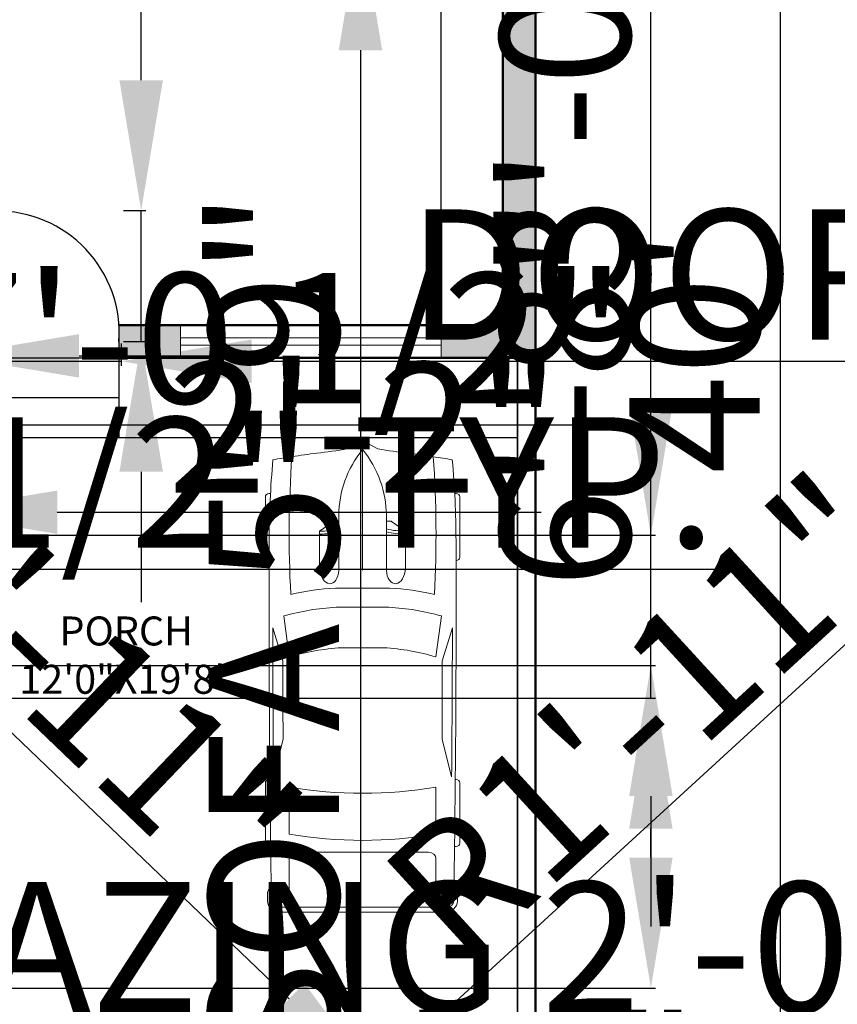
# Model space of a CAD drawing. Units: inches. Extents: x -299 to 1164, y -2 to 940.
# Tile 6 of 11: x 597 to 822, y 218 to 490. Entities that reach past the tile are written whole.
import ezdxf

# ---------------------------------------------------------------- set-up
doc = ezdxf.new("R2010")
doc.units = ezdxf.units.IN
for name, color, linetype, lineweight in [('A-AREA-IDEN', 3, 'Continuous', 25), ('C-SITE-VEHL', 8, 'Continuous', 13), ('C-SITE-WALL', 7, 'Continuous', 35), ('dimensions', 191, 'Continuous', 18), ('doors', 20, 'Continuous', 25), ('outer walls', 7, 'Continuous', 50), ('stairs', 6, 'Continuous', 25), ('windows', 130, 'Continuous', 18)]:
    doc.layers.add(name, color=color, linetype=linetype, lineweight=lineweight)
doc.layers.add('A-WALL-PATT', color=240, linetype='Continuous', lineweight=13, true_color=0xed1f24)
doc.styles.get("Standard").update_dxf_attribs({"font": 'arial.ttf'})
doc.dimstyles.new('ISO-25', dxfattribs={"dimtxt": 36, "dimasz": 36, "dimexe": 1.25, "dimexo": 0.625, "dimtad": 1, "dimlunit": 3, "dimtxsty": 'Standard', "dimcen": 2.5, "dimazin": 0, "dimtfac": 1, "dimtmove": 0, "dimatfit": 3, "dimfxl": 1, "dimarcsym": 0})

# ---------------------------------------------------------------- blocks, each defined once
blk = doc.blocks.new('*U11')
for p, q in [((536, 950.2), (536, 935.5)), ((1182.5, 987.8), (567.7, 987.8)), ((1214.1, 949.7), (1214.1, 950.2)), ((2234.8, 809.5), (1898.9, 912.4)), ((3411.6, 904.3), (3029.9, 807.2)), ((3440.5, 941.7), (3440.5, 950.2)), ((3472.1, 987.8), (4086.9, 987.8)), ((4118.5, 950.2), (4118.5, 934.1)), ((1778.8, 801), (2194.7, 745.5)), ((4736.4, -850.9), (4736.4, 850.9)), ((4785.3, -832.1), (4785.3, 832.1)), ((3515.9, 745.5), (3994.1, 745.5)), ((4736.4, 745.5), (4242, 745.5)), ((4178.7, 670.3), (4178.7, -670.3)), ((819.6, 295.3), (917.7, 436.1)), ((917.7, 436.1), (1293.8, 436.1)), ((756.2, 241.4), (1312.8, 241.4)), ((815.9, 241.4), (815.9, 283.3)), ((1496.5, -273.7), (1496.5, 273.7)), ((1690.4, -267.4), (1690.4, 267.4)), ((2101.5, 215.8), (2101.5, -215.8)), ((4736.4, -267.4), (4736.4, 267.4)), ((83, 155.7), (2.6, 10.3)), ((0, 0), (1312.8, 0)), ((2.6, -10.3), (83, -155.7)), ((756.2, -241.4), (1312.8, -241.4)), ((815.9, -241.4), (815.9, -283.3)), ((819.6, -295.3), (917.7, -436.1)), ((917.7, -436.1), (1293.8, -436.1)), ((2194.7, -745.5), (1778.8, -801)), ((3994.1, -745.5), (3515.9, -745.5)), ((4242, -745.5), (4736.4, -745.5)), ((2234.8, -809.5), (1898.9, -912.4)), ((3411.6, -904.3), (3029.9, -807.2)), ((536, -950.2), (536, -935.5)), ((1182.5, -987.8), (567.7, -987.8)), ((1214.1, -949.7), (1214.1, -950.2)), ((3440.5, -941.7), (3440.5, -950.2)), ((3472.1, -987.8), (4086.9, -987.8)), ((4118.5, -950.2), (4118.5, -934.1))]:
    blk.add_line(p, q)
for centre, major_axis, ratio, start_param, end_param in [((6757.2, -699.1), (0, 7958), 0.842304, 1.367076, 1.39176), ((1046.3, -12467.9), (0, 13417.1), 0.842304, 0.00281, 0.075598), ((567.7, 950.2), (0, -37.6), 0.842304, 3.141593, 4.712389), ((1637.8, -268112.7), (0, 269062.9), 0.842304, -0.013397, 0.002797), ((1182.5, 950.2), (0, 37.6), 0.842304, -1.570796, 0), ((1637.8, -268112.7), (0, -269025.3), 0.842304, 3.133765, 3.140441), ((3472.1, 950.2), (0, -37.6), 0.842304, 3.141593, 4.712389), ((4086.9, 950.2), (0, 37.6), 0.842304, -1.570796, 0), ((4588, 910.3), (0, 56.4), 0.842304, -0.013017, 1.249894), ((1637.8, -268131.5), (0, 269121), 0.842304, -0.013397, -0.013017), ((4673.1, 850.9), (0, -75.2), 0.842304, 1.570796, 3.128196), ((4673.1, 832.1), (0, -133.3), 0.842304, 1.570796, 3.128196), ((3436.4, 136.8), (0, 2077), 0.842304, 1.245306, 1.50788), ((2433, -93125.4), (0, -93935.2), 0.842304, 3.134049, 3.144098), ((6583, -699.1), (0, -7754.7), 0.842304, 4.528606, 4.561838), ((951.8, -15086.6), (0, -15832.5), 0.842304, 3.096046, 3.200911), ((3413.8, 136.8), (0, -2280.3), 0.842304, 4.449482, 4.652344), ((3799.7, 71.1), (0, -2021.3), 0.842304, 4.372215, 4.640744), ((433.9, 0), (0, 3734.3), 0.842304, 4.511394, 4.913384), ((912, 0), (0, 3734.3), 0.842304, 4.511394, 4.913384), ((4242, 670.3), (0, 75.2), 0.842304, 0, 1.570796), ((-5194.2, 1330.9), (0, -6374.4), 0.842304, 1.385369, 1.434372), ((331.1, 432), (0, 696.4), 0.842304, 4.435146, 4.718221), ((360.7, 432), (0, 696.4), 0.842304, 4.435146, 4.718221), ((1290.1, 338.8), (161, -9.1), 0.603834, -1.395552, 1.581315), ((756.2, -1185.2), (0, 1426.7), 0.842304, 0, 0.590319), ((831.8, 283.3), (0, 18.8), 0.842304, 0.879714, 1.570796), ((15.8, 0), (0, -18.8), 0.842304, 4.131459, 5.293319), ((756.2, 1185.2), (0, 1426.7), 0.842304, 2.551274, 3.141593), ((-5194.2, -1330.9), (0, 6374.4), 0.842304, -1.434372, -1.385369), ((831.8, -283.3), (0, -18.8), 0.842304, 4.712389, 5.403472), ((331.1, -432), (0, -696.4), 0.842304, 1.564964, 1.848039), ((360.7, -432), (0, -696.4), 0.842304, 1.564964, 1.848039), ((3413.8, -136.8), (0, -2280.3), 0.842304, -1.510751, -1.307889), ((3436.4, -136.8), (0, -2077), 0.842304, -1.50788, -1.245306), ((3799.7, -71.1), (0, -2021.3), 0.842304, -1.499151, -1.230623), ((6583, 699.1), (0, 7754.7), 0.842304, 1.721348, 1.754579), ((4242, -670.3), (0, -75.2), 0.842304, 4.712389, 6.283185), ((6757.2, 699.1), (0, 7958), 0.842304, 1.749832, 1.774517), ((951.8, 15086.6), (0, -15832.5), 0.842304, -0.059319, 0.045547), ((2433, 93125.4), (0, -93935.2), 0.842304, -0.002505, 0.007544), ((4673.1, -850.9), (0, 75.2), 0.842304, 3.15499, 4.712389), ((4673.1, -832.1), (0, -133.3), 0.842304, 0.013397, 1.570796), ((1046.3, 12467.9), (0, -13417.1), 0.842304, -0.075598, -0.00281), ((567.7, -950.2), (0, 37.6), 0.842304, 1.570796, 3.141593), ((1637.8, 268112.7), (0, 269062.9), 0.842304, 3.138796, 3.15499), ((1182.5, -950.2), (0, -37.6), 0.842304, 0, 1.570796), ((1637.8, 268112.7), (0, -269025.3), 0.842304, 0.001152, 0.007828), ((3472.1, -950.2), (0, -37.6), 0.842304, -1.570796, 0), ((4086.9, -950.2), (0, 37.6), 0.842304, 3.141593, 4.712389), ((4588, -910.3), (0, -56.4), 0.842304, -1.249894, 0.013017), ((1637.8, 268131.5), (0, 269121), 0.842304, 3.15461, 3.15499)]:
    blk.add_ellipse(centre, major_axis=major_axis, ratio=ratio, start_param=start_param, end_param=end_param)
at = {"extrusion": (0, 0, -1)}
blk.add_ellipse((1290.1, -338.8), major_axis=(161, 9.1), ratio=0.603834, start_param=-1.395552, end_param=1.581315, dxfattribs=at)
blk = doc.blocks.new('*D14')
at = {"layer": 'Defpoints', "color": 0, "transparency": 16777216}
for p in [(739.07, 638.49), (739.07, 158.49), (806.66, 158.49)]:
    blk.add_point(p, dxfattribs=at)
at = {"layer": 'dimensions', "color": 0, "lineweight": -2, "transparency": 16777216}
for p, q in [((739.7, 638.49), (807.91, 638.49)), ((806.66, 602.49), (806.66, 194.49)), ((739.7, 158.49), (807.91, 158.49))]:
    blk.add_line(p, q, dxfattribs=at)
at = {"layer": 'dimensions', "color": 0, "transparency": 16777216}
for points in [[(800.66, 602.49), (812.66, 602.49), (806.66, 638.49)], [(800.66, 194.49), (812.66, 194.49), (806.66, 158.49)]]:
    blk.add_solid(points, dxfattribs=at)
at = {"layer": 'dimensions', "color": 0, "transparency": 16777216, "insert": (787.65, 398.49), "char_height": 36, "attachment_point": 5, "rotation": 90}
blk.add_mtext("40'", dxfattribs=at)
blk = doc.blocks.new('WIN-72IN')
for p, q in [((0, 5.5), (72, 5.5)), ((0, 3.5), (72, 3.5))]:
    blk.add_line(p, q)
blk.add_lwpolyline([(0, 0), (72, 0), (72, 9), (0, 9)], close=True)
blk = doc.blocks.new('DOOR-36IN')
blk.add_lwpolyline([(0, 36), (2, 36), (2, 0), (0, 0)], close=True)
blk.add_arc((2.32, 2.25), 33.75, 356.1776, 90.5492)
blk = doc.blocks.new('*D23')
at = {"layer": 'Defpoints', "color": 0, "transparency": 16777216}
for p in [(701.12, 586.52), (690.74, 517.34), (701.12, 517.34)]:
    blk.add_point(p, dxfattribs=at)
at = {"layer": 'dimensions', "color": 0, "lineweight": -2, "transparency": 16777216}
for p, q in [((690.74, 622.52), (690.74, 658.52)), ((700.49, 586.52), (689.49, 586.52)), ((690.74, 586.52), (690.74, 517.34)), ((700.49, 517.34), (689.49, 517.34)), ((690.74, 481.34), (690.74, 197.66))]:
    blk.add_line(p, q, dxfattribs=at)
at = {"layer": 'dimensions', "color": 0, "transparency": 16777216}
for points in [[(684.74, 622.52), (696.74, 622.52), (690.74, 586.52)], [(684.74, 481.34), (696.74, 481.34), (690.74, 517.34)]]:
    blk.add_solid(points, dxfattribs=at)
at = {"layer": 'dimensions', "color": 0, "transparency": 16777216, "insert": (671.49, 321.5), "char_height": 36, "attachment_point": 5, "rotation": 90}
blk.add_mtext('SOFA 5\'-9"', dxfattribs=at)
blk = doc.blocks.new('*D28')
at = {"layer": 'Defpoints', "color": 0, "transparency": 16777216}
for p in [(379.74, 342.99), (412.07, 342.99), (412.07, 338.11)]:
    blk.add_point(p, dxfattribs=at)
at = {"layer": 'dimensions', "color": 0, "lineweight": -2, "transparency": 16777216}
for p, q in [((379.74, 342.36), (379.74, 336.86)), ((412.07, 342.36), (412.07, 336.86)), ((343.74, 338.11), (307.74, 338.11)), ((379.74, 338.11), (412.07, 338.11)), ((448.07, 338.11), (789.26, 338.11))]:
    blk.add_line(p, q, dxfattribs=at)
at = {"layer": 'dimensions', "color": 0, "transparency": 16777216}
for points in [[(343.74, 344.11), (343.74, 332.11), (379.74, 338.11)], [(448.07, 344.11), (448.07, 332.11), (412.07, 338.11)]]:
    blk.add_solid(points, dxfattribs=at)
at = {"layer": 'dimensions', "color": 0, "transparency": 16777216, "insert": (636.66, 357.35), "char_height": 36, "attachment_point": 5}
blk.add_mtext('2\'-8 1/2" TYP.', dxfattribs=at)
blk = doc.blocks.new('*D29')
at = {"layer": 'Defpoints', "color": 0, "transparency": 16777216}
for p in [(304.07, 183.49), (376.07, 183.49), (376.07, 172.69)]:
    blk.add_point(p, dxfattribs=at)
at = {"layer": 'dimensions', "color": 0, "lineweight": -2, "transparency": 16777216}
for p, q in [((304.07, 182.86), (304.07, 171.44)), ((376.07, 182.86), (376.07, 171.44)), ((268.07, 172.69), (232.07, 172.69)), ((304.07, 172.69), (376.07, 172.69)), ((412.07, 172.69), (904.87, 172.69))]:
    blk.add_line(p, q, dxfattribs=at)
at = {"layer": 'dimensions', "color": 0, "transparency": 16777216}
for points in [[(268.07, 178.69), (268.07, 166.69), (304.07, 172.69)], [(412.07, 178.69), (412.07, 166.69), (376.07, 172.69)]]:
    blk.add_solid(points, dxfattribs=at)
at = {"layer": 'dimensions', "color": 0, "transparency": 16777216, "insert": (676.47, 191.94), "char_height": 36, "attachment_point": 5}
blk.add_mtext('WINDOW 6\'-0" TYP.', dxfattribs=at)
blk = doc.blocks.new('*D33')
at = {"layer": 'Defpoints', "color": 0, "transparency": 16777216}
for p in [(419.84, 213.49), (443.84, 213.49), (443.84, 209.89)]:
    blk.add_point(p, dxfattribs=at)
at = {"layer": 'dimensions', "color": 0, "lineweight": -2, "transparency": 16777216}
for p, q in [((419.84, 212.86), (419.84, 208.64)), ((443.84, 212.86), (443.84, 208.64)), ((383.84, 209.89), (347.84, 209.89)), ((419.84, 209.89), (443.84, 209.89)), ((479.84, 209.89), (970.68, 209.89))]:
    blk.add_line(p, q, dxfattribs=at)
at = {"layer": 'dimensions', "color": 0, "transparency": 16777216}
for points in [[(383.84, 215.89), (383.84, 203.89), (419.84, 209.89)], [(479.84, 215.89), (479.84, 203.89), (443.84, 209.89)]]:
    blk.add_solid(points, dxfattribs=at)
at = {"layer": 'dimensions', "color": 0, "transparency": 16777216, "insert": (743.26, 229.13), "char_height": 36, "attachment_point": 5}
blk.add_mtext('GLAZING 2\'-0" TYP.', dxfattribs=at)
blk = doc.blocks.new('*D35')
at = {"layer": 'Defpoints', "color": 0, "transparency": 16777216}
for p in [(307.07, 495.34), (268.07, 489.49), (307.07, 489.49)]:
    blk.add_point(p, dxfattribs=at)
at = {"layer": 'dimensions', "color": 0, "lineweight": -2, "transparency": 16777216}
for p, q in [((232.07, 495.34), (196.07, 495.34)), ((268.07, 490.11), (268.07, 496.59)), ((268.07, 495.34), (307.07, 495.34)), ((307.07, 490.11), (307.07, 496.59)), ((343.07, 495.34), (749.73, 495.34))]:
    blk.add_line(p, q, dxfattribs=at)
at = {"layer": 'dimensions', "color": 0, "transparency": 16777216}
for points in [[(232.07, 501.34), (232.07, 489.34), (268.07, 495.34)], [(343.07, 501.34), (343.07, 489.34), (307.07, 495.34)]]:
    blk.add_solid(points, dxfattribs=at)
at = {"layer": 'dimensions', "color": 0, "transparency": 16777216, "insert": (564.4, 514.36), "char_height": 36, "attachment_point": 5}
blk.add_mtext('VENT 3\'-3" TYP.', dxfattribs=at)
blk = doc.blocks.new('*D37')
at = {"layer": 'Defpoints', "color": 0, "transparency": 16777216}
for p in [(588.07, 400.99), (624.7, 400.99), (624.7, 395.5)]:
    blk.add_point(p, dxfattribs=at)
at = {"layer": 'dimensions', "color": 0, "lineweight": -2, "transparency": 16777216}
for p, q in [((588.07, 400.36), (588.07, 394.25)), ((624.7, 400.36), (624.7, 394.25)), ((552.07, 395.5), (516.07, 395.5)), ((588.07, 395.5), (624.7, 395.5)), ((660.7, 395.5), (1164.33, 395.5))]:
    blk.add_line(p, q, dxfattribs=at)
at = {"layer": 'dimensions', "color": 0, "transparency": 16777216}
for points in [[(552.07, 401.5), (552.07, 389.5), (588.07, 395.5)], [(660.7, 401.5), (660.7, 389.5), (624.7, 395.5)]]:
    blk.add_solid(points, dxfattribs=at)
at = {"layer": 'dimensions', "color": 0, "transparency": 16777216, "insert": (930.51, 414.76), "char_height": 36, "attachment_point": 5}
blk.add_mtext('DOOR 3\'-0 1/2" TYP.', dxfattribs=at)
blk = doc.blocks.new('*D38')
at = {"layer": 'Defpoints', "color": 0, "transparency": 16777216}
for p in [(624.7, 437.08), (630.19, 437.08), (624.7, 400.99)]:
    blk.add_point(p, dxfattribs=at)
at = {"layer": 'dimensions', "color": 0, "lineweight": -2, "transparency": 16777216}
for p, q in [((630.19, 473.08), (630.19, 729.74)), ((625.32, 437.08), (631.44, 437.08)), ((630.19, 400.99), (630.19, 437.08)), ((625.32, 400.99), (631.44, 400.99)), ((630.19, 364.99), (630.19, 328.99))]:
    blk.add_line(p, q, dxfattribs=at)
at = {"layer": 'dimensions', "color": 0, "transparency": 16777216}
for points in [[(624.19, 473.08), (636.19, 473.08), (630.19, 437.08)], [(624.19, 364.99), (636.19, 364.99), (630.19, 400.99)]]:
    blk.add_solid(points, dxfattribs=at)
at = {"layer": 'dimensions', "color": 0, "transparency": 16777216, "insert": (611.17, 619.41), "char_height": 36, "attachment_point": 5, "rotation": 90}
blk.add_mtext('3\'-0" TYP.', dxfattribs=at)
blk = doc.blocks.new('*D39')
at = {"layer": 'Defpoints', "color": 0, "transparency": 16777216}
for p in [(575.6, 509.45), (484.6, 495.8), (575.6, 495.8)]:
    blk.add_point(p, dxfattribs=at)
at = {"layer": 'dimensions', "color": 0, "lineweight": -2, "transparency": 16777216}
for p, q in [((484.6, 496.43), (484.6, 510.7)), ((520.6, 509.45), (539.6, 509.45)), ((575.6, 496.43), (575.6, 510.7)), ((575.6, 509.45), (1008.53, 509.45))]:
    blk.add_line(p, q, dxfattribs=at)
at = {"layer": 'dimensions', "color": 0, "transparency": 16777216}
for points in [[(520.6, 515.45), (520.6, 503.45), (484.6, 509.45)], [(539.6, 515.45), (539.6, 503.45), (575.6, 509.45)]]:
    blk.add_solid(points, dxfattribs=at)
at = {"layer": 'dimensions', "color": 0, "transparency": 16777216, "insert": (810.07, 528.69), "char_height": 36, "attachment_point": 5}
blk.add_mtext('DINING SET 7\'-7"', dxfattribs=at)
blk = doc.blocks.new('*D42')
at = {"layer": 'Defpoints', "color": 0, "transparency": 16777216}
for p in [(545.04, 358.33), (571.04, 358.33), (571.04, 353.83)]:
    blk.add_point(p, dxfattribs=at)
at = {"layer": 'dimensions', "color": 0, "lineweight": -2, "transparency": 16777216}
for p, q in [((545.04, 357.71), (545.04, 352.58)), ((571.04, 357.71), (571.04, 352.58)), ((509.04, 353.83), (473.04, 353.83)), ((545.04, 353.83), (571.04, 353.83)), ((607.04, 353.83), (740.6, 353.83))]:
    blk.add_line(p, q, dxfattribs=at)
at = {"layer": 'dimensions', "color": 0, "transparency": 16777216}
for points in [[(509.04, 359.83), (509.04, 347.83), (545.04, 353.83)], [(607.04, 359.83), (607.04, 347.83), (571.04, 353.83)]]:
    blk.add_solid(points, dxfattribs=at)
at = {"layer": 'dimensions', "color": 0, "transparency": 16777216, "insert": (691.82, 372.53), "char_height": 36, "attachment_point": 5}
blk.add_mtext('2\'-2"', dxfattribs=at)
blk = doc.blocks.new('*D46')
at = {"layer": 'Defpoints', "color": 0, "transparency": 16777216}
for p in [(579.07, 302.49), (770.93, 302.49), (579.07, 222.49)]:
    blk.add_point(p, dxfattribs=at)
at = {"layer": 'dimensions', "color": 0, "lineweight": -2, "transparency": 16777216}
for p, q in [((770.93, 302.49), (770.93, 435.63)), ((579.7, 302.49), (772.18, 302.49)), ((770.93, 258.49), (770.93, 266.49)), ((579.7, 222.49), (772.18, 222.49))]:
    blk.add_line(p, q, dxfattribs=at)
at = {"layer": 'dimensions', "color": 0, "transparency": 16777216}
for points in [[(764.93, 266.49), (776.93, 266.49), (770.93, 302.49)], [(764.93, 258.49), (776.93, 258.49), (770.93, 222.49)]]:
    blk.add_solid(points, dxfattribs=at)
at = {"layer": 'dimensions', "color": 0, "transparency": 16777216, "insert": (751.92, 387.06), "char_height": 36, "attachment_point": 5, "rotation": 90}
blk.add_mtext('6\'-8"', dxfattribs=at)
blk = doc.blocks.new('*D47')
at = {"layer": 'Defpoints', "color": 0, "transparency": 16777216}
for p in [(502.07, 668.99), (466.07, 222.49), (502.07, 222.49)]:
    blk.add_point(p, dxfattribs=at)
at = {"layer": 'dimensions', "color": 0, "lineweight": -2, "transparency": 16777216}
for p, q in [((430.07, 668.99), (394.07, 668.99)), ((466.07, 223.11), (466.07, 670.24)), ((466.07, 668.99), (502.07, 668.99)), ((502.07, 223.11), (502.07, 670.24)), ((538.07, 668.99), (670.99, 668.99))]:
    blk.add_line(p, q, dxfattribs=at)
at = {"layer": 'dimensions', "color": 0, "transparency": 16777216}
for points in [[(430.07, 674.99), (430.07, 662.99), (466.07, 668.99)], [(538.07, 674.99), (538.07, 662.99), (502.07, 668.99)]]:
    blk.add_solid(points, dxfattribs=at)
at = {"layer": 'dimensions', "color": 0, "transparency": 16777216, "insert": (622.53, 688.01), "char_height": 36, "attachment_point": 5}
blk.add_mtext('3\'-0"', dxfattribs=at)
blk = doc.blocks.new('*D48')
at = {"layer": 'Defpoints', "color": 0, "transparency": 16777216}
for p in [(546.07, 668.99), (535.07, 222.49), (546.07, 222.49)]:
    blk.add_point(p, dxfattribs=at)
at = {"layer": 'dimensions', "color": 0, "lineweight": -2, "transparency": 16777216}
for p, q in [((499.07, 668.99), (463.07, 668.99)), ((535.07, 223.11), (535.07, 670.24)), ((535.07, 668.99), (546.07, 668.99)), ((546.07, 223.11), (546.07, 670.24)), ((582.07, 668.99), (742.99, 668.99))]:
    blk.add_line(p, q, dxfattribs=at)
at = {"layer": 'dimensions', "color": 0, "transparency": 16777216}
for points in [[(499.07, 674.99), (499.07, 662.99), (535.07, 668.99)], [(582.07, 674.99), (582.07, 662.99), (546.07, 668.99)]]:
    blk.add_solid(points, dxfattribs=at)
at = {"layer": 'dimensions', "color": 0, "transparency": 16777216, "insert": (680.53, 687.99), "char_height": 36, "attachment_point": 5}
blk.add_mtext('0\'-11"', dxfattribs=at)
blk = doc.blocks.new('*D51')
at = {"layer": 'Defpoints', "color": 0, "transparency": 16777216}
for p in [(739.07, 668.99), (713.07, 405.49), (739.07, 396.49)]:
    blk.add_point(p, dxfattribs=at)
at = {"layer": 'dimensions', "color": 0, "lineweight": -2, "transparency": 16777216}
for p, q in [((677.07, 668.99), (641.07, 668.99)), ((713.07, 406.11), (713.07, 670.24)), ((713.07, 668.99), (739.07, 668.99)), ((739.07, 397.11), (739.07, 670.24)), ((775.07, 668.99), (908.63, 668.99))]:
    blk.add_line(p, q, dxfattribs=at)
at = {"layer": 'dimensions', "color": 0, "transparency": 16777216}
for points in [[(677.07, 674.99), (677.07, 662.99), (713.07, 668.99)], [(775.07, 674.99), (775.07, 662.99), (739.07, 668.99)]]:
    blk.add_solid(points, dxfattribs=at)
at = {"layer": 'dimensions', "color": 0, "transparency": 16777216, "insert": (859.85, 687.69), "char_height": 36, "attachment_point": 5}
blk.add_mtext('2\'-2"', dxfattribs=at)
blk = doc.blocks.new('*D52')
at = {"layer": 'Defpoints', "color": 0, "transparency": 16777216}
for p in [(575.54, 668.99), (527.54, 311.49), (575.54, 311.49)]:
    blk.add_point(p, dxfattribs=at)
at = {"layer": 'dimensions', "color": 0, "lineweight": -2, "transparency": 16777216}
for p, q in [((491.54, 668.99), (455.54, 668.99)), ((527.54, 312.11), (527.54, 670.24)), ((527.54, 668.99), (575.54, 668.99)), ((575.54, 312.11), (575.54, 670.24)), ((611.54, 668.99), (745.94, 668.99))]:
    blk.add_line(p, q, dxfattribs=at)
at = {"layer": 'dimensions', "color": 0, "transparency": 16777216}
for points in [[(491.54, 674.99), (491.54, 662.99), (527.54, 668.99)], [(611.54, 674.99), (611.54, 662.99), (575.54, 668.99)]]:
    blk.add_solid(points, dxfattribs=at)
at = {"layer": 'dimensions', "color": 0, "transparency": 16777216, "insert": (696.74, 687.99), "char_height": 36, "attachment_point": 5}
blk.add_mtext('4\'-0"', dxfattribs=at)
blk = doc.blocks.new('*D56')
at = {"layer": 'Defpoints', "color": 0, "transparency": 16777216}
for p in [(541.07, 377.99), (456.35, 347.49), (541.07, 347.49)]:
    blk.add_point(p, dxfattribs=at)
at = {"layer": 'dimensions', "color": 0, "lineweight": -2, "transparency": 16777216}
for p, q in [((456.35, 348.11), (456.35, 379.24)), ((492.35, 377.99), (505.07, 377.99)), ((541.07, 348.11), (541.07, 379.24)), ((541.07, 377.99), (757.61, 377.99))]:
    blk.add_line(p, q, dxfattribs=at)
at = {"layer": 'dimensions', "color": 0, "transparency": 16777216}
for points in [[(492.35, 383.99), (492.35, 371.99), (456.35, 377.99)], [(505.07, 383.99), (505.07, 371.99), (541.07, 377.99)]]:
    blk.add_solid(points, dxfattribs=at)
at = {"layer": 'dimensions', "color": 0, "transparency": 16777216, "insert": (667.34, 397.23), "char_height": 36, "attachment_point": 5}
blk.add_mtext('7\'-0 1/2"', dxfattribs=at)
blk = doc.blocks.new('*D57')
at = {"layer": 'Defpoints', "color": 0, "transparency": 16777216}
for p in [(541.07, 427.49), (577.07, 427.49), (541.07, 396.99)]:
    blk.add_point(p, dxfattribs=at)
at = {"layer": 'dimensions', "color": 0, "lineweight": -2, "transparency": 16777216}
for p, q in [((541.07, 426.86), (541.07, 395.74)), ((577.07, 426.86), (577.07, 395.74)), ((505.07, 396.99), (372.15, 396.99)), ((577.07, 396.99), (541.07, 396.99)), ((613.07, 396.99), (649.07, 396.99))]:
    blk.add_line(p, q, dxfattribs=at)
at = {"layer": 'dimensions', "color": 0, "transparency": 16777216}
for points in [[(505.07, 402.99), (505.07, 390.99), (541.07, 396.99)], [(613.07, 402.99), (613.07, 390.99), (577.07, 396.99)]]:
    blk.add_solid(points, dxfattribs=at)
at = {"layer": 'dimensions', "color": 0, "transparency": 16777216, "insert": (420.61, 416.01), "char_height": 36, "attachment_point": 5}
blk.add_mtext('3\'-0"', dxfattribs=at)
blk = doc.blocks.new('*D58')
at = {"layer": 'Defpoints', "color": 0, "transparency": 16777216}
for p in [(456.35, 347.49), (770.93, 347.49), (456.35, 311.49)]:
    blk.add_point(p, dxfattribs=at)
at = {"layer": 'dimensions', "color": 0, "lineweight": -2, "transparency": 16777216}
for p, q in [((770.93, 383.49), (770.93, 516.41)), ((456.97, 347.49), (772.18, 347.49)), ((770.93, 311.49), (770.93, 347.49)), ((456.97, 311.49), (772.18, 311.49)), ((770.93, 275.49), (770.93, 239.49))]:
    blk.add_line(p, q, dxfattribs=at)
at = {"layer": 'dimensions', "color": 0, "transparency": 16777216}
for points in [[(764.93, 383.49), (776.93, 383.49), (770.93, 347.49)], [(764.93, 275.49), (776.93, 275.49), (770.93, 311.49)]]:
    blk.add_solid(points, dxfattribs=at)
at = {"layer": 'dimensions', "color": 0, "transparency": 16777216, "insert": (751.91, 467.95), "char_height": 36, "attachment_point": 5, "rotation": 90}
blk.add_mtext('3\'-0"', dxfattribs=at)
blk = doc.blocks.new('*D59')
at = {"layer": 'Defpoints', "color": 0, "transparency": 16777216}
for p in [(697.05, 194.59), (730.81, 162.24)]:
    blk.add_point(p, dxfattribs=at)
at = {"layer": 'dimensions', "color": 0, "lineweight": -2, "transparency": 16777216}
for p, q in [((530.01, 354.68), (671.06, 219.5)), ((730.81, 162.24), (697.05, 194.59))]:
    blk.add_line(p, q, dxfattribs=at)
at = {"layer": 'dimensions', "color": 0, "transparency": 16777216}
blk.add_solid([(675.21, 223.83), (666.91, 215.17), (697.05, 194.59)], dxfattribs=at)
at = {"layer": 'dimensions', "color": 0, "transparency": 16777216, "insert": (600.7, 313.27), "char_height": 36, "attachment_point": 5, "rotation": 316.2186}
blk.add_mtext('R3\'-11"', dxfattribs=at)
blk = doc.blocks.new('*D60')
at = {"layer": 'Defpoints', "color": 0, "transparency": 16777216}
for p in [(672.12, 177.62), (655.34, 162.24)]:
    blk.add_point(p, dxfattribs=at)
at = {"layer": 'dimensions', "color": 0, "lineweight": -2, "transparency": 16777216}
for p, q in [((842.68, 333.96), (698.66, 201.95)), ((655.34, 162.24), (672.12, 177.62))]:
    blk.add_line(p, q, dxfattribs=at)
at = {"layer": 'dimensions', "color": 0, "transparency": 16777216}
blk.add_solid([(694.61, 206.37), (702.71, 197.52), (672.12, 177.62)], dxfattribs=at)
at = {"layer": 'dimensions', "color": 0, "transparency": 16777216, "insert": (771.3, 293.9), "char_height": 36, "attachment_point": 5, "rotation": 42.5105}
blk.add_mtext('R1\'-11"', dxfattribs=at)
blk = doc.blocks.new('*D62')
at = {"layer": 'Defpoints', "color": 0, "transparency": 16777216}
for p in [(420.34, 307.74), (441.36, 288.12)]:
    blk.add_point(p, dxfattribs=at)
at = {"layer": 'dimensions', "color": 0, "lineweight": -2, "transparency": 16777216}
for p, q in [((420.34, 307.74), (441.36, 288.12)), ((646.59, 96.57), (467.68, 263.55))]:
    blk.add_line(p, q, dxfattribs=at)
at = {"layer": 'dimensions', "color": 0, "transparency": 16777216}
blk.add_solid([(471.78, 267.94), (463.59, 259.17), (441.36, 288.12)], dxfattribs=at)
at = {"layer": 'dimensions', "color": 0, "transparency": 16777216, "insert": (583.27, 181.68), "char_height": 36, "attachment_point": 5, "rotation": 316.9755}
blk.add_mtext('3X R2\'-5"', dxfattribs=at)

msp = doc.modelspace()

# ---------------------------------------------------------------- hatches: boundary and pattern name
at = {"layer": 'A-WALL-PATT'}
h = msp.add_hatch(color=256, dxfattribs=at)
h.dxf.hatch_style = 1
h.paths.add_polyline_path([(312.071, 460.489), (307.071, 460.489), (307.071, 432.489), (307.071, 427.489), (372.071, 427.489), (372.071, 375.489), (372.071, 370.489), (380.071, 370.489, -0.0217424), (380.071, 372.989), (380.071, 375.489), (377.071, 375.489), (377.071, 427.489), (417.071, 427.489), (417.071, 489.489), (412.071, 489.489), (412.071, 484.489), (412.071, 432.489), (312.071, 432.489)], flags=17)
h.paths.add_polyline_path([(340.071, 372.989, -0.0217424), (340.071, 375.489), (268.071, 375.489), (268.071, 427.489), (268.071, 432.489), (268.071, 484.489), (268.071, 489.489), (268.071, 629.489), (412.071, 629.489), (412.071, 527.563, -0.0185322), (414.571, 527.489), (417.071, 527.489), (417.071, 629.489), (581.071, 629.489), (581.071, 553.489), (586.071, 553.489), (586.071, 629.489), (730.071, 629.489), (730.071, 405.489), (713.071, 405.489), (713.071, 396.489), (739.071, 396.489), (739.071, 638.489), (259.071, 638.489), (259.071, 183.489), (304.071, 183.489), (304.071, 192.489), (268.071, 192.489), (268.071, 370.489), (340.071, 370.489)])
h.paths.add_polyline_path([(417.071, 188.489), (417.071, 213.489), (461.071, 213.489), (461.071, 188.489)], flags=16)
h.paths.add_polyline_path([(586.071, 313.578), (577.071, 313.578), (577.071, 311.489), (575.54, 311.489), (575.54, 302.489), (586.071, 302.489)], flags=16)
h.paths.add_polyline_path([(586.071, 405.489), (586.071, 481.489), (581.071, 481.489), (581.071, 432.489), (499.071, 432.489), (499.071, 427.489), (577.071, 427.489), (577.071, 385.578), (586.071, 385.578), (586.071, 396.489)], flags=17)
h.paths.add_polyline_path([(641.071, 405.489), (624.071, 405.489, -0.0333689), (624.071, 400.989), (624.071, 396.489), (641.071, 396.489)], flags=17)
h.paths.add_polyline_path([(491.866, 222.489), (491.866, 213.489), (586.071, 213.489), (586.071, 222.489)])
edge = h.paths.add_edge_path()
edge.add_line((467.866, 213.489), (467.866, 222.489))
edge.add_line((467.866, 222.489), (466.071, 222.489))
edge.add_line((466.071, 222.489), (466.071, 302.489))
edge.add_line((466.071, 302.489), (527.54, 302.489))
edge.add_line((527.54, 302.489), (527.54, 311.489))
edge.add_line((527.54, 311.489), (449.071, 311.489))
edge.add_line((449.071, 311.489), (449.071, 308.989))
edge.add_arc((420.339, 307.739), 28.759, -2.4911, 2.4911, ccw=False)
edge.add_line((449.071, 306.489), (461.071, 306.489))
edge.add_line((461.071, 306.489), (461.071, 222.489))
edge.add_line((461.071, 222.489), (443.844, 222.489))
edge.add_line((443.844, 222.489), (443.844, 213.489))
edge.add_line((443.844, 213.489), (419.844, 213.489))
edge.add_line((419.844, 213.489), (419.844, 222.489))
edge.add_line((419.844, 222.489), (417.071, 222.489))
edge.add_line((417.071, 222.489), (417.071, 306.489))
edge.add_line((417.071, 306.489), (417.071, 311.489))
edge.add_line((417.071, 311.489), (417.071, 375.489))
edge.add_line((417.071, 375.489), (412.071, 375.489))
edge.add_line((412.071, 375.489), (412.071, 370.489))
edge.add_line((412.071, 370.489), (412.071, 192.489))
edge.add_line((412.071, 192.489), (376.071, 192.489))
edge.add_line((376.071, 192.489), (376.071, 183.489))
edge.add_line((376.071, 183.489), (412.071, 183.489))
edge.add_line((412.071, 183.489), (466.071, 183.489))
edge.add_line((466.071, 183.489), (466.071, 213.489))
edge.add_line((466.071, 213.489), (467.866, 213.489))

# ---------------------------------------------------------------- linework, layer by layer
at = {"layer": 'C-SITE-WALL'}
msp.add_line((734.071, 163.489), (734.071, 396.489), dxfattribs=at)
at = {"layer": 'doors'}
msp.add_line((624.071, 405.489), (624.071, 396.489), dxfattribs=at)
at = {"layer": 'outer walls'}
for p, q in [((739.071, 158.489), (739.071, 638.489)), ((730.071, 405.489), (730.071, 629.489)), ((730.071, 405.489), (624.071, 405.489)), ((739.071, 396.489), (624.071, 396.489))]:
    msp.add_line(p, q, dxfattribs=at)
at = {"layer": 'stairs'}
for p, q in [((588.071, 396.489), (624.071, 396.489)), ((624.071, 396.489), (624.071, 374.489)), ((586.071, 385.489), (624.071, 385.489)), ((586.071, 374.489), (624.071, 374.489)), ((624.071, 374.489), (734.071, 374.489))]:
    msp.add_line(p, q, dxfattribs=at)

# ---------------------------------------------------------------- block references
at = {"layer": 'C-SITE-VEHL', "xscale": 0.0271817845741683, "yscale": 0.0271817845741683, "zscale": 0.0271817845741683, "rotation": 270}
msp.add_blockref('*U11', (691.331, 373.539), dxfattribs=at)
at = {"layer": 'doors'}
msp.add_blockref('DOOR-36IN', (588.071, 400.989), dxfattribs=at)
at = {"layer": 'windows'}
msp.add_blockref('WIN-72IN', (641.071, 396.489), dxfattribs=at)

# ---------------------------------------------------------------- texts
at = {"layer": 'A-AREA-IDEN', "insert": (591.141, 325.046), "char_height": 8, "attachment_point": 1}
msp.add_mtext_dynamic_manual_height_columns('\\pxqc,t15;PORCH\\P12\'0"X19\'8"', width=69.83809, gutter_width=12.5, heights=[0], dxfattribs=at)

# ---------------------------------------------------------------- dimensions: what is measured, and where the dimension line sits
at = {"layer": 'dimensions'}
for base, p1, p2, angle, text, picture, middle in [((630.192, 437.079), (624.698, 400.989), (624.698, 437.079), 90, '<> TYP.', '*D38', (611.174, 619.411)), ((690.742, 517.338), (701.119, 586.518), (701.119, 517.338), 270, 'SOFA <>', '*D23', (671.49, 321.5))]:
    dim = msp.add_linear_dim(base=base, p1=p1, p2=p2, angle=angle, text=text, dimstyle='ISO-25', override={"dimdec": 1, "dimlfac": 1, "dimrnd": 0, "dimzin": 1, "dimdsep": 46, "dimlunit": 4, "dimfrac": 2}, dxfattribs=at)
    dim.commit()
    dim.dimension.update_dxf_attribs({"geometry": picture, "text_midpoint": middle})
for base, p1, p2, picture, middle in [((502.071, 668.989), (466.071, 222.489), (502.071, 222.489), '*D47', (622.532, 688.007)), ((575.54, 668.989), (527.54, 311.489), (575.54, 311.489), '*D52', (696.738, 687.995)), ((546.071, 668.989), (535.071, 222.489), (546.071, 222.489), '*D48', (680.53, 687.995)), ((739.071, 668.989), (713.071, 405.489), (739.071, 396.489), '*D51', (859.852, 687.688)), ((541.071, 377.989), (456.348, 347.489), (541.071, 347.489), '*D56', (667.34, 397.228)), ((571.036, 353.835), (545.036, 358.335), (571.036, 358.335), '*D42', (691.817, 372.534))]:
    dim = msp.add_linear_dim(base=base, p1=p1, p2=p2, dimstyle='ISO-25', override={"dimdec": 1, "dimlfac": 1, "dimrnd": 0, "dimzin": 1, "dimdsep": 46, "dimlunit": 4, "dimfrac": 2}, dxfattribs=at)
    dim.commit()
    dim.dimension.update_dxf_attribs({"geometry": picture, "text_midpoint": middle})
for base, p1, p2, angle, override, picture, middle in [((806.659, 158.489), (739.071, 638.489), (739.071, 158.489), 90, {"dimclrd": 0, "dimclre": 0, "dimclrt": 0}, '*D14', (787.654, 398.489)), ((770.929, 347.489), (456.348, 311.489), (456.348, 347.489), 90, {"dimdec": 1, "dimlfac": 1, "dimrnd": 0, "dimzin": 1, "dimdsep": 46, "dimlunit": 4, "dimfrac": 2}, '*D58', (751.911, 467.95)), ((541.071, 396.989), (577.071, 427.489), (541.071, 427.489), 180, {"dimdec": 1, "dimlfac": 1, "dimrnd": 0, "dimzin": 1, "dimdsep": 46, "dimlunit": 4, "dimfrac": 2}, '*D57', (420.61, 416.007)), ((770.929, 302.489), (579.071, 222.489), (579.071, 302.489), 90, {"dimdec": 1, "dimlfac": 1, "dimrnd": 0, "dimzin": 1, "dimdsep": 46, "dimlunit": 4, "dimfrac": 2}, '*D46', (751.923, 387.061))]:
    dim = msp.add_linear_dim(base=base, p1=p1, p2=p2, angle=angle, dimstyle='ISO-25', override=override, dxfattribs=at)
    dim.commit()
    dim.dimension.update_dxf_attribs({"geometry": picture, "text_midpoint": middle})
for base, p1, p2, text, picture, middle in [((575.6, 509.45), (484.6, 495.8), (575.6, 495.8), 'DINING SET <>', '*D39', (810.066, 528.689)), ((307.071, 495.339), (268.071, 489.489), (307.071, 489.489), 'VENT <> TYP.', '*D35', (564.399, 514.357)), ((624.698, 395.495), (588.071, 400.989), (624.698, 400.989), 'DOOR <> TYP.', '*D37', (930.512, 414.759)), ((412.071, 338.114), (379.736, 342.989), (412.071, 342.989), '<> TYP.', '*D28', (636.665, 357.353)), ((443.844, 209.889), (419.844, 213.489), (443.844, 213.489), 'GLAZING <> TYP.', '*D33', (743.261, 229.128)), ((376.071, 172.689), (304.071, 183.489), (376.071, 183.489), 'WINDOW <> TYP.', '*D29', (676.471, 191.94))]:
    dim = msp.add_linear_dim(base=base, p1=p1, p2=p2, text=text, dimstyle='ISO-25', override={"dimdec": 1, "dimlfac": 1, "dimrnd": 0, "dimzin": 1, "dimdsep": 46, "dimlunit": 4, "dimfrac": 2}, dxfattribs=at)
    dim.commit()
    dim.dimension.update_dxf_attribs({"geometry": picture, "text_midpoint": middle})
for center, mpoint, picture, middle in [((730.81, 162.239), (697.053, 194.59), '*D59', (600.698, 313.273)), ((655.344, 162.239), (672.123, 177.62), '*D60', (771.303, 293.901))]:
    dim = msp.add_radius_dim(center=center, mpoint=mpoint, dimstyle='ISO-25', override={"dimdec": 1, "dimlfac": 1, "dimrnd": 0, "dimzin": 1, "dimdsep": 46, "dimlunit": 4, "dimfrac": 2}, dxfattribs=at)
    dim.commit()
    dim.dimension.update_dxf_attribs({"geometry": picture, "text_midpoint": middle})
dim = msp.add_radius_dim(center=(420.339, 307.739), mpoint=(441.364, 288.116), text='3X <>', dimstyle='ISO-25', override={"dimdec": 1, "dimlfac": 1, "dimrnd": 0, "dimzin": 1, "dimdsep": 46, "dimlunit": 4, "dimfrac": 2}, dxfattribs=at)
dim.commit()
dim.dimension.update_dxf_attribs({"geometry": '*D62', "text_midpoint": (583.273, 181.684)})

doc.saveas('drawing.dxf')
